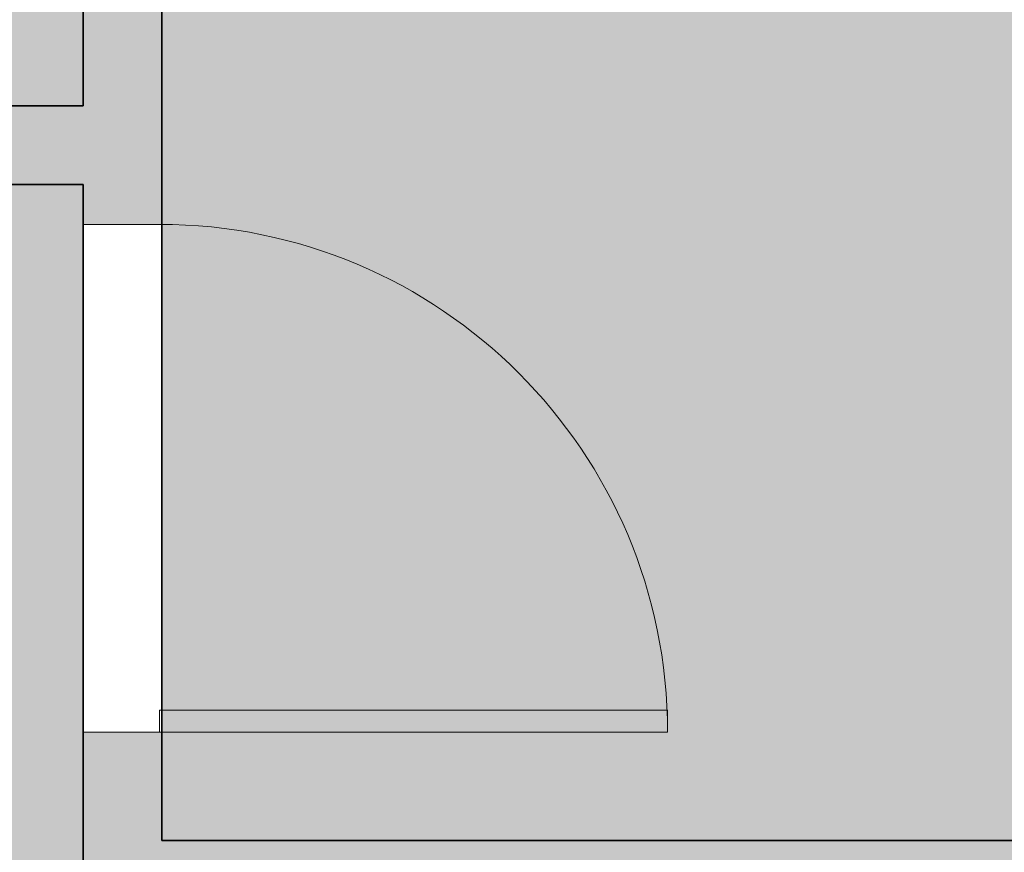
# Model space of a CAD drawing. Units: inches. Extents: x 1316 to 1777, y 813 to 1650.
# Tile 18 of 22: x 1567 to 1623, y 1434 to 1481. Entities that reach past the tile are written whole.
import ezdxf

# ---------------------------------------------------------------- set-up
doc = ezdxf.new("R2010")
doc.units = ezdxf.units.IN
doc.header["$MEASUREMENT"] = 0
for name, color, linetype, lineweight in [('A-DOOR', 4, 'Continuous', 18), ('A-WALL-PATT', 250, 'Continuous', 13), ('walls', 250, 'Continuous', 35)]:
    doc.layers.add(name, color=color, linetype=linetype, lineweight=lineweight)
doc.layers.add('A-FLOR-PATT', color=254, linetype='Continuous', lineweight=13, true_color=0xfeeab9)

# ---------------------------------------------------------------- blocks, each defined once
blk = doc.blocks.new('*U15')
for p, q in [((0, 0), (0, -6)), ((40, 0), (40, -6))]:
    blk.add_line(p, q)
blk.add_lwpolyline([(0, 0), (0, 40), (1.75, 40), (1.75, 0)], close=True)
blk.add_arc((0, 0), 40, 0, 90)

msp = doc.modelspace()

# ---------------------------------------------------------------- hatches: boundary and pattern name
at = {"layer": 'A-FLOR-PATT'}
h = msp.add_hatch(color=256, dxfattribs=at)
h.dxf.hatch_style = 1
h.paths.add_polyline_path([(1704.173, 1566.369), (1574.845, 1566.369), (1574.845, 1434.369), (1704.173, 1434.369)])
h.paths.add_polyline_path([(1630.932, 1542.856), (1660.956, 1542.856), (1660.956, 1535.716), (1688.427, 1535.716), (1688.322, 1546.604), (1686.085, 1547.859), (1686.091, 1547.88), (1685.166, 1550.963), (1681.619, 1555.397), (1678.246, 1552.474), (1678.253, 1552.433), (1678.187, 1552.423), (1681.619, 1555.397), (1683.601, 1556.058), (1683.639, 1556.172), (1683.764, 1556.112), (1686.94, 1557.171), (1688.039, 1558.585), (1688.034, 1558.699), (1688.108, 1558.672), (1686.969, 1557.208), (1686.965, 1557.18), (1681.619, 1555.397), (1682.039, 1554.872), (1682.12, 1554.846), (1682.107, 1554.788), (1685.145, 1550.989), (1685.188, 1550.977), (1685.173, 1550.941), (1685.764, 1548.971), (1688.364, 1547.814), (1702.185, 1547.814), (1702.301, 1535.716), (1702.301, 1481.716), (1702.418, 1469.617), (1688.544, 1469.617), (1688.427, 1481.716), (1660.956, 1481.716), (1660.956, 1470.853), (1630.932, 1470.853)], flags=16)
h.paths.add_polyline_path([(1624.931, 1450.279), (1703.919, 1450.279), (1703.919, 1436.32), (1703.919, 1435.026), (1624.931, 1435.026), (1624.931, 1435.469)], flags=16)
h.paths.add_polyline_path([(1624.931, 1443.714), (1625.995, 1443.714), (1625.995, 1449.229), (1626.752, 1449.229), (1626.752, 1443.714), (1628.114, 1443.714), (1628.114, 1449.229), (1628.871, 1449.229), (1628.871, 1443.714), (1630.502, 1443.714), (1630.502, 1449.229), (1631.259, 1449.229), (1631.259, 1443.714), (1632.968, 1443.714), (1632.968, 1449.229), (1633.724, 1449.229), (1633.724, 1443.714), (1638.318, 1443.714), (1641.013, 1449.6), (1641.689, 1449.29), (1639.136, 1443.714), (1640.128, 1443.714), (1642.823, 1449.6), (1643.499, 1449.29), (1640.945, 1443.714), (1642.323, 1443.714), (1645.018, 1449.6), (1645.694, 1449.29), (1643.141, 1443.714), (1647.035, 1443.714), (1647.035, 1449.229), (1647.792, 1449.229), (1647.792, 1443.714), (1649.606, 1443.714), (1649.606, 1449.229), (1650.363, 1449.229), (1650.363, 1443.714), (1652.865, 1443.714), (1652.865, 1449.229), (1653.621, 1449.229), (1653.621, 1443.714), (1657.035, 1443.714), (1657.035, 1449.229), (1657.792, 1449.229), (1657.792, 1443.714), (1660.083, 1443.714), (1660.083, 1449.229), (1660.839, 1449.229), (1660.839, 1443.714), (1662.605, 1443.714), (1662.605, 1449.229), (1663.362, 1449.229), (1663.362, 1443.714), (1667.702, 1443.714), (1667.702, 1449.229), (1668.459, 1449.229), (1668.459, 1443.714), (1671.655, 1443.714), (1670.316, 1449.229), (1671.051, 1449.407), (1672.434, 1443.714), (1679.696, 1443.714), (1680.179, 1449.244), (1680.933, 1449.178), (1680.455, 1443.714), (1683.5, 1443.714), (1682.225, 1448.723), (1682.959, 1448.91), (1684.281, 1443.714), (1688.219, 1443.714), (1688.219, 1449.229), (1688.976, 1449.229), (1688.976, 1443.714), (1690.482, 1443.714), (1690.482, 1449.229), (1691.239, 1449.229), (1691.239, 1443.714), (1692.488, 1443.714), (1692.488, 1449.229), (1693.245, 1449.229), (1693.245, 1443.714), (1695.009, 1443.714), (1695.009, 1449.229), (1695.766, 1449.229), (1695.766, 1443.714), (1701.029, 1443.714), (1700.875, 1443.379), (1695.766, 1443.379), (1695.766, 1435.872), (1695.009, 1435.872), (1695.009, 1443.379), (1693.245, 1443.379), (1693.245, 1435.872), (1692.488, 1435.872), (1692.488, 1443.379), (1691.239, 1443.379), (1691.239, 1435.872), (1690.482, 1435.872), (1690.482, 1443.379), (1688.976, 1443.379), (1688.976, 1435.872), (1688.219, 1435.872), (1688.219, 1443.379), (1684.366, 1443.379), (1686.252, 1435.965), (1685.518, 1435.779), (1683.585, 1443.379), (1680.426, 1443.379), (1679.77, 1435.872), (1679.016, 1435.938), (1679.666, 1443.379), (1677.602, 1443.379), (1677.602, 1435.46), (1676.845, 1435.46), (1676.845, 1443.379), (1672.515, 1443.379), (1674.202, 1436.427), (1673.467, 1436.249), (1671.736, 1443.379), (1668.459, 1443.379), (1668.459, 1435.872), (1667.702, 1435.872), (1667.702, 1443.379), (1663.362, 1443.379), (1663.362, 1435.872), (1662.605, 1435.872), (1662.605, 1443.379), (1660.839, 1443.379), (1660.839, 1435.872), (1660.083, 1435.872), (1660.083, 1443.379), (1657.792, 1443.379), (1657.792, 1435.872), (1657.035, 1435.872), (1657.035, 1443.379), (1653.621, 1443.379), (1653.621, 1435.872), (1652.865, 1435.872), (1652.865, 1443.379), (1650.363, 1443.379), (1650.363, 1435.872), (1649.606, 1435.872), (1649.606, 1443.379), (1647.792, 1443.379), (1647.792, 1435.872), (1647.035, 1435.872), (1647.035, 1443.379), (1642.988, 1443.379), (1639.39, 1435.522), (1638.715, 1435.832), (1642.17, 1443.379), (1640.792, 1443.379), (1637.195, 1435.522), (1636.519, 1435.832), (1639.974, 1443.379), (1638.983, 1443.379), (1635.385, 1435.522), (1634.709, 1435.832), (1638.165, 1443.379), (1633.724, 1443.379), (1633.724, 1435.872), (1632.968, 1435.872), (1632.968, 1443.379), (1631.259, 1443.379), (1631.259, 1435.872), (1630.502, 1435.872), (1630.502, 1443.379), (1628.871, 1443.379), (1628.871, 1435.872), (1628.114, 1435.872), (1628.114, 1443.379), (1626.752, 1443.379), (1626.752, 1435.872), (1625.995, 1435.872), (1625.995, 1443.379), (1624.931, 1443.379)], flags=0)
h.paths.add_polyline_path([(1683.839, 1491.517), (1691.022, 1491.517), (1691.071, 1491.582), (1691.071, 1529.618), (1699.231, 1529.618), (1699.231, 1513.795), (1691.071, 1513.795), (1691.071, 1507.34), (1699.231, 1507.34), (1699.231, 1491.517), (1691.022, 1491.517), (1683.839, 1481.774)], flags=0)
h.paths.add_polyline_path([(1691.015, 1475.341, -1), (1699.947, 1475.341, -1)], flags=0)
h.paths.add_polyline_path([(1690.898, 1541.439, -1), (1699.83, 1541.439, -1)], flags=0)
h.paths.add_polyline_path([(1505.845, 1469.591), (1505.845, 1566.369), (1386.064, 1566.369), (1386.064, 1450.329), (1465.697, 1450.329), (1465.697, 1449.245), (1466.177, 1449.025), (1465.697, 1447.977), (1465.697, 1436.055), (1465.697, 1434.369), (1505.845, 1434.369), (1505.845, 1440.551), (1476.949, 1440.551), (1476.949, 1441.822), (1476.977, 1441.822, -0.400014)])
edge = h.paths.add_edge_path(flags=16)
edge.add_spline(control_points=[(1456.973, 1471.794), (1457.023, 1471.721), (1457.138, 1471.554), (1456.942, 1471.242), (1456.67, 1470.851), (1456.943, 1470.632), (1457.081, 1470.522)], knot_values=[0, 0, 0, 0, 0.352144, 0.802463, 1.439322, 2.0926, 2.0926, 2.0926, 2.0926], degree=3, periodic=0)
edge.add_spline(control_points=[(1457.325, 1471.794), (1457.375, 1471.721), (1457.49, 1471.554), (1457.294, 1471.242), (1457.022, 1470.851), (1457.295, 1470.632), (1457.433, 1470.522)], knot_values=[0, 0, 0, 0, 0.352144, 0.802463, 1.439322, 2.0926, 2.0926, 2.0926, 2.0926], degree=3, periodic=0)
edge = h.paths.add_edge_path(flags=16)
edge.add_line((1429.513, 1471.794), (1429.513, 1482.657))
edge.add_line((1429.513, 1482.657), (1402.042, 1482.657))
edge.add_line((1402.042, 1482.657), (1401.925, 1470.559))
edge.add_line((1401.925, 1470.559), (1388.051, 1470.559))
edge.add_line((1388.051, 1470.559), (1388.167, 1482.657))
edge.add_line((1388.167, 1482.657), (1388.167, 1536.657))
edge.add_line((1388.167, 1536.657), (1388.284, 1548.755))
edge.add_line((1388.284, 1548.755), (1402.158, 1548.755))
edge.add_line((1402.158, 1548.755), (1402.042, 1536.657))
edge.add_line((1402.042, 1536.657), (1429.513, 1536.657))
edge.add_line((1429.513, 1536.657), (1429.513, 1543.797))
edge.add_line((1429.513, 1543.797), (1456.932, 1543.797))
edge.add_spline(control_points=[(1456.932, 1543.797), (1456.987, 1543.874), (1457.108, 1544.044), (1456.911, 1544.361), (1456.638, 1544.752), (1456.911, 1544.971), (1457.049, 1545.082)], knot_values=[0, 0, 0, 0, 0.373994, 0.824314, 1.461173, 2.114451, 2.114451, 2.114451, 2.114451], degree=3, periodic=0)
edge.add_spline(control_points=[(1457.401, 1545.082), (1457.263, 1544.971), (1456.99, 1544.752), (1457.263, 1544.361), (1457.46, 1544.044), (1457.339, 1543.874), (1457.284, 1543.797)], knot_values=[0, 0, 0, 0, 0.653278, 1.290138, 1.740457, 2.114451, 2.114451, 2.114451, 2.114451], degree=3, periodic=0)
edge.add_line((1457.284, 1543.797), (1459.536, 1543.797))
edge.add_line((1459.536, 1543.797), (1459.536, 1471.794))
edge.add_line((1459.536, 1471.794), (1429.513, 1471.794))
h.paths.add_polyline_path([(1406.63, 1482.715), (1399.446, 1492.458), (1399.398, 1492.458), (1391.238, 1492.458), (1391.238, 1508.281), (1399.398, 1508.281), (1399.398, 1514.736), (1391.238, 1514.736), (1391.238, 1530.559), (1399.398, 1530.559), (1399.398, 1492.524), (1399.446, 1492.458), (1406.63, 1492.458)], flags=0)
h.paths.add_polyline_path([(1399.454, 1476.282, -1), (1390.522, 1476.282, -1)], flags=0)
h.paths.add_polyline_path([(1390.638, 1542.38, -1), (1399.571, 1542.38, -1)], flags=0)
h.paths.add_polyline_path([(1487.293, 1548.286), (1487.08, 1548.252), (1487.104, 1547.964)], flags=16)
h.paths.add_polyline_path([(1491.493, 1552.843), (1490.887, 1552.654), (1490.949, 1552.372)], flags=16)
h.paths.add_polyline_path([(1489.966, 1554.409), (1489.859, 1554.561), (1489.718, 1554.445)], flags=16)
h.paths.add_polyline_path([(1497.301, 1546.483), (1497.294, 1546.462), (1497.309, 1546.453)], flags=16)
h.paths.add_polyline_path([(1496.386, 1549.553), (1492.828, 1554), (1492.655, 1554.939), (1492.454, 1555.029), (1492.589, 1555.296), (1491.806, 1559.547), (1491.869, 1559.506), (1491.824, 1559.451), (1492.828, 1554), (1494.81, 1554.661), (1494.848, 1554.774), (1494.973, 1554.715), (1496.01, 1555.061), (1496.078, 1555.314), (1496.341, 1555.171), (1498.15, 1555.774), (1499.249, 1557.187), (1499.243, 1557.301), (1499.317, 1557.275), (1498.179, 1555.811), (1498.174, 1555.782), (1492.828, 1554), (1493.249, 1553.474), (1493.33, 1553.449), (1493.316, 1553.39), (1495.203, 1551.032), (1495.702, 1550.957), (1495.574, 1550.568), (1496.354, 1549.592), (1496.397, 1549.58)], flags=16)
h.paths.add_polyline_path([(1486.021, 1555.224), (1485.958, 1555.549), (1483.595, 1557.912), (1483.28, 1557.859), (1483.243, 1558.264), (1486.27, 1555.237)], flags=16)
h.paths.add_polyline_path([(1505.845, 1469.591, 0.400014), (1476.977, 1441.822), (1505.845, 1441.822)], flags=17)
h = msp.add_hatch(color=256, dxfattribs=at)
h.dxf.hatch_style = 1
h.paths.add_polyline_path([(1561.016, 1510.243), (1561.016, 1510.275), (1562.477, 1510.275), (1562.477, 1476.879), (1562.477, 1471.869), (1529.081, 1471.869), (1529.081, 1476.879, -0.401453)])
h.paths.add_polyline_path([(1570.345, 1566.369), (1510.345, 1566.369), (1510.345, 1502.159), (1526.605, 1502.159), (1526.605, 1480.004), (1510.345, 1480.004), (1510.345, 1476.369), (1529.081, 1476.369), (1529.081, 1476.879, -0.401453), (1561.016, 1510.243), (1561.016, 1510.275), (1562.477, 1510.275), (1562.477, 1476.369), (1570.345, 1476.369)])
h.paths.add_polyline_path([(1528.659, 1540.982), (1528.659, 1542.825), (1529.12, 1552.041), (1528.659, 1552.041), (1528.659, 1553.884), (1529.12, 1553.884, -0.206081), (1535.571, 1559.041), (1535.571, 1561.257), (1534.65, 1561.257), (1534.65, 1562.179), (1532.806, 1562.179), (1532.806, 1563.1), (1543.866, 1563.1), (1543.866, 1562.179), (1542.023, 1562.179), (1542.023, 1561.257), (1541.101, 1561.257), (1541.101, 1559.041, -0.206081), (1547.552, 1553.884), (1548.013, 1553.884), (1548.013, 1552.041), (1547.552, 1552.041), (1547.552, 1542.825), (1548.013, 1542.825), (1548.013, 1540.982)], flags=16)
h.paths.add_polyline_path([(1704.173, 1429.869), (1602.173, 1429.869), (1602.173, 1408.281), (1631.07, 1408.281), (1631.07, 1407.011), (1631.042, 1407.011, -0.400014), (1602.173, 1379.241), (1602.173, 1369.869), (1625.31, 1369.869), (1625.31, 1385.783), (1647.465, 1385.783), (1647.465, 1369.869), (1704.173, 1369.869)])
h.paths.add_polyline_path([(1669.737, 1382.593), (1670.237, 1382.593), (1670.237, 1392.593), (1669.737, 1392.593), (1669.737, 1394.593), (1690.737, 1394.593), (1690.737, 1392.593), (1690.237, 1392.593), (1690.237, 1382.593), (1690.737, 1382.593), (1690.737, 1380.593), (1690.237, 1380.593, -0.206081), (1683.237, 1374.997), (1683.237, 1372.593), (1684.237, 1372.593), (1684.237, 1371.593), (1686.237, 1371.593), (1686.237, 1370.593), (1674.237, 1370.593), (1674.237, 1371.593), (1676.237, 1371.593), (1676.237, 1372.593), (1677.237, 1372.593), (1677.237, 1374.997, -0.206081), (1670.237, 1380.593), (1669.737, 1380.593)], flags=16)
h.paths.add_polyline_path([(1631.042, 1407.011), (1602.029, 1407.011), (1602.029, 1408.281), (1597.673, 1408.281), (1597.673, 1379.241), (1602.029, 1379.241, 0.401453)])
h = msp.add_hatch(color=256, dxfattribs=at)
h.dxf.hatch_style = 1
h.paths.add_polyline_path([(1567.673, 1281.369), (1651.673, 1281.369), (1651.673, 1365.369), (1597.673, 1365.369), (1597.673, 1429.869), (1570.345, 1429.869), (1570.345, 1471.869), (1510.345, 1471.869), (1510.345, 1429.869), (1444.564, 1429.869), (1444.564, 1322.882), (1444.564, 1300.088), (1510.564, 1300.088), (1510.564, 1295.094), (1510.564, 1240.869), (1386.064, 1240.869), (1386.064, 1171.185), (1400.961, 1171.185), (1400.961, 1106.742), (1386.064, 1106.742), (1386.064, 1072.869), (1510.564, 1072.869), (1510.564, 1040.173), (1541.068, 1040.173, -0.367085), (1572.764, 1069.547), (1572.764, 1069.579), (1574.225, 1069.579), (1574.225, 1040.173), (1616.037, 1040.173), (1616.037, 1086.627), (1616.037, 1103.705), (1613.066, 1105.235), (1616.037, 1106.686), (1616.037, 1123.869), (1567.673, 1123.869)])
h.paths.add_polyline_path([(1508.987, 1198.018), (1511.117, 1198.018), (1511.117, 1200.148), (1532.595, 1200.148), (1532.595, 1198.018), (1534.725, 1198.018), (1534.725, 1176.008), (1530.465, 1176.008), (1530.465, 1176.718), (1513.247, 1176.718), (1513.247, 1176.008), (1508.987, 1176.008)], flags=16)
h.paths.add_polyline_path([(1505.979, 1151.315), (1521.504, 1151.315), (1521.504, 1123.623), (1505.979, 1123.623)], flags=16)
h.paths.add_polyline_path([(1507.734, 1150.101, -1), (1506.932, 1150.101, -1)], flags=0)
h.paths.add_polyline_path([(1512.288, 1138.353), (1512.28, 1138.392), (1512.219, 1138.376)], flags=0)
h.paths.add_polyline_path([(1511.539, 1138.926), (1511.802, 1138.967), (1511.817, 1139.27), (1511.607, 1139.246)], flags=0)
h.paths.add_polyline_path([(1513.745, 1140.234), (1513.68, 1139.885), (1514.014, 1140.045), (1513.855, 1140.308)], flags=0)
h.paths.add_polyline_path([(1513.759, 1139.089), (1514.005, 1139.255), (1513.807, 1139.483), (1513.564, 1139.327)], flags=0)
h.paths.add_polyline_path([(1514.219, 1138.385), (1514.336, 1138.33), (1514.544, 1138.32), (1514.802, 1138.874), (1514.451, 1138.716)], flags=0)
h.paths.add_polyline_path([(1514.577, 1137.439), (1514.573, 1137.4), (1514.699, 1137.4), (1514.696, 1137.402)], flags=0)
h.paths.add_polyline_path([(1512.26, 1136.199), (1512.199, 1136.399), (1512.032, 1136.325), (1512.095, 1136.101), (1512.257, 1136.192)], flags=0)
h.paths.add_polyline_path([(1512.644, 1137.274), (1512.356, 1137.23), (1512.432, 1137.049), (1512.703, 1137.093)], flags=0)
h.paths.add_polyline_path([(1513.049, 1137.593), (1512.979, 1137.8), (1512.843, 1137.757), (1512.887, 1137.556)], flags=0)
h.paths.add_polyline_path([(1513.269, 1138.556), (1513.571, 1137.962), (1513.459, 1136.814), (1513.212, 1137.878), (1513.032, 1138.443)], flags=0)
h.paths.add_polyline_path([(1514.891, 1136.377), (1514.696, 1136.401), (1514.683, 1136.246), (1514.87, 1136.165)], flags=0)
h.paths.add_polyline_path([(1514.142, 1137.293), (1514.047, 1136.743), (1514.27, 1136.751), (1514.328, 1137.265)], flags=0)
h.paths.add_polyline_path([(1515.362, 1138.976), (1515.334, 1138.638), (1515.596, 1138.588), (1515.627, 1138.932)], flags=0)
h.paths.add_polyline_path([(1537.285, 1177.912), (1537.995, 1177.912), (1537.995, 1195.13), (1537.285, 1195.13), (1537.285, 1199.39), (1559.295, 1199.39), (1559.295, 1197.26), (1561.425, 1197.26), (1561.425, 1175.782), (1559.295, 1175.782), (1559.295, 1173.652), (1559.379, 1173.652), (1559.379, 1171.514), (1561.517, 1171.514), (1561.517, 1098.819), (1559.379, 1098.819), (1559.379, 1096.68), (1537.285, 1096.68), (1537.285, 1100.957), (1537.997, 1100.957), (1537.997, 1169.376), (1537.285, 1169.376), (1537.285, 1173.652)], flags=16)
h.paths.add_polyline_path([(1518.623, 1345.565), (1519.133, 1345.48), (1519.133, 1345.485), (1518.623, 1345.567)], flags=16)
h.paths.add_polyline_path([(1518.798, 1374.15), (1519.308, 1374.064), (1519.308, 1374.069), (1518.798, 1374.152)], flags=16)
h.paths.add_polyline_path([(1537.764, 1413.501), (1537.678, 1412.991), (1537.683, 1412.991), (1537.766, 1413.501)], flags=16)
h.paths.add_polyline_path([(1572.905, 1373.821), (1573.927, 1373.975), (1574.027, 1390.309), (1573.007, 1390.475), (1573.007, 1390.475)], flags=16)
h.paths.add_polyline_path([(1572.73, 1345.237), (1573.752, 1345.39), (1573.852, 1361.724), (1572.832, 1361.89), (1572.832, 1361.89)], flags=16)
h.paths.add_polyline_path([(1537.211, 1322.643), (1537.364, 1321.621), (1553.698, 1321.521), (1553.864, 1322.541)], flags=16)
h.paths.add_polyline_path([(1535.908, 1331.328), (1527.214, 1331.382), (1527.664, 1404.885), (1564.416, 1404.66), (1563.966, 1331.157), (1555.273, 1331.21), (1553.947, 1323.051), (1537.134, 1323.154)], flags=16)
h.paths.add_polyline_path([(1536.15, 1336.503), (1536.235, 1337.572), (1536.323, 1338.628), (1536.411, 1339.663), (1536.495, 1340.67), (1536.574, 1341.66), (1536.648, 1342.648), (1536.717, 1343.649), (1536.78, 1344.678), (1536.837, 1345.75), (1536.913, 1347.475), (1536.93, 1348.082), (1536.867, 1346.314), (1536.754, 1344.188), (1536.619, 1342.219), (1536.495, 1340.67), (1536.411, 1339.663), (1536.323, 1338.628), (1536.235, 1337.572), (1536.15, 1336.503), (1536.071, 1335.432), (1536.002, 1334.37), (1535.917, 1332.754), (1535.909, 1332.308), (1535.964, 1333.78), (1536.071, 1335.432)], flags=0)
h.paths.add_polyline_path([(1540.412, 1338.345), (1540.539, 1339.037), (1540.667, 1339.758), (1540.798, 1340.518), (1540.93, 1341.325), (1541.063, 1342.187), (1541.196, 1343.109), (1541.326, 1344.085), (1541.45, 1345.102), (1541.566, 1346.15), (1541.669, 1347.219), (1541.758, 1348.296), (1541.829, 1349.371), (1541.879, 1350.434), (1541.906, 1351.476), (1541.91, 1352.5), (1541.895, 1353.512), (1541.861, 1354.518), (1541.812, 1355.524), (1541.749, 1356.537), (1541.674, 1357.561), (1541.551, 1359.062), (1541.495, 1359.67), (1541.589, 1358.603), (1541.721, 1356.977), (1541.846, 1354.98), (1541.912, 1352.982), (1541.903, 1350.951), (1541.806, 1348.87), (1541.628, 1346.713), (1541.396, 1344.612), (1541.135, 1342.656), (1540.872, 1340.947), (1540.617, 1339.466), (1540.412, 1338.345), (1540.288, 1337.675), (1540.166, 1337.018), (1540.049, 1336.365), (1539.937, 1335.71), (1539.837, 1335.055), (1539.758, 1334.403), (1539.709, 1333.756), (1539.697, 1333.12), (1539.751, 1332.162), (1539.822, 1331.89), (1539.691, 1332.775), (1539.714, 1334.035), (1539.867, 1335.303), (1540.085, 1336.577), (1540.288, 1337.675)], flags=0)
h.paths.add_polyline_path([(1545.599, 1331.584), (1545.601, 1331.617), (1545.614, 1331.689), (1545.737, 1332.197), (1545.767, 1332.332), (1545.84, 1332.681), (1545.925, 1333.114), (1546.016, 1333.614), (1546.108, 1334.164), (1546.196, 1334.748), (1546.276, 1335.349), (1546.342, 1335.952), (1546.388, 1336.539), (1546.412, 1337.098), (1546.414, 1337.632), (1546.395, 1338.145), (1546.359, 1338.645), (1546.306, 1339.137), (1546.24, 1339.627), (1546.161, 1340.121), (1546.073, 1340.625), (1545.888, 1341.63), (1545.718, 1342.621), (1545.547, 1343.945), (1545.432, 1345.534), (1545.404, 1347.402), (1545.418, 1348.013), (1545.411, 1346.957), (1545.425, 1345.988), (1545.463, 1345.105), (1545.521, 1344.301), (1545.596, 1343.566), (1545.683, 1342.892), (1545.778, 1342.27), (1545.877, 1341.691), (1545.977, 1341.145), (1546.133, 1340.297), (1546.327, 1339.075), (1546.434, 1337.615), (1546.377, 1336.279), (1546.246, 1335.079), (1546.032, 1333.665), (1545.84, 1332.681), (1545.767, 1332.332)], flags=0)
h.paths.add_polyline_path([(1551.803, 1337.656), (1551.963, 1338.25), (1552.102, 1338.801), (1552.225, 1339.338), (1552.331, 1339.865), (1552.418, 1340.377), (1552.487, 1340.873), (1552.536, 1341.348), (1552.563, 1341.801), (1552.569, 1342.228), (1552.551, 1342.627), (1552.51, 1342.995), (1552.446, 1343.333), (1552.363, 1343.646), (1552.261, 1343.937), (1552.144, 1344.207), (1552.012, 1344.461), (1551.868, 1344.7), (1551.746, 1344.882), (1550.887, 1346.052), (1550.428, 1347.126), (1550.183, 1348.353), (1550.048, 1349.632), (1549.978, 1351.224), (1549.974, 1353.141), (1549.989, 1353.748), (1549.975, 1352.682), (1549.977, 1351.708), (1549.996, 1350.825), (1550.031, 1350.027), (1550.082, 1349.31), (1550.15, 1348.669), (1550.234, 1348.098), (1550.335, 1347.593), (1550.452, 1347.149), (1550.584, 1346.76), (1550.73, 1346.419), (1550.887, 1346.117), (1551.05, 1345.848), (1551.217, 1345.602), (1551.386, 1345.372), (1551.553, 1345.151), (1552, 1344.537), (1552.454, 1343.495), (1552.591, 1342.266), (1552.509, 1340.905), (1552.246, 1339.367), (1551.925, 1338.101), (1551.619, 1336.984), (1551.406, 1336.2), (1551.01, 1334.699), (1550.877, 1334.155), (1551.264, 1335.677), (1551.619, 1336.984)], flags=0)
h.paths.add_polyline_path([(1558.642, 1348.348), (1558.795, 1348.811), (1558.918, 1349.215), (1559.008, 1349.575), (1559.061, 1349.904), (1559.076, 1350.214), (1559.054, 1350.506), (1559.001, 1350.776), (1558.919, 1351.021), (1558.814, 1351.239), (1558.688, 1351.425), (1558.546, 1351.578), (1558.392, 1351.694), (1558.229, 1351.772), (1558.059, 1351.812), (1557.882, 1351.819), (1557.701, 1351.794), (1557.515, 1351.742), (1557.327, 1351.665), (1557.136, 1351.566), (1556.944, 1351.448), (1556.752, 1351.315), (1556.742, 1351.307), (1556.175, 1350.878), (1555.982, 1350.741), (1555.79, 1350.618), (1555.103, 1350.248), (1554.019, 1350.696), (1553.658, 1351.734), (1553.592, 1352.861), (1553.705, 1354.248), (1553.753, 1354.657), (1553.685, 1354.004), (1553.638, 1353.425), (1553.615, 1352.918), (1553.615, 1352.476), (1553.637, 1352.094), (1553.681, 1351.766), (1553.745, 1351.485), (1553.828, 1351.246), (1553.929, 1351.043), (1554.048, 1350.87), (1554.182, 1350.722), (1554.33, 1350.599), (1554.491, 1350.501), (1554.662, 1350.43), (1554.841, 1350.388), (1555.026, 1350.374), (1555.215, 1350.39), (1555.406, 1350.437), (1555.598, 1350.514), (1555.79, 1350.618), (1555.982, 1350.741), (1556.175, 1350.878), (1556.367, 1351.024), (1556.559, 1351.171), (1556.752, 1351.315), (1556.944, 1351.448), (1557.136, 1351.566), (1557.327, 1351.665), (1558.043, 1351.957), (1558.894, 1351.316), (1559.137, 1350.09), (1558.886, 1349.087), (1558.642, 1348.348), (1558.463, 1347.812), (1558.261, 1347.187), (1558.039, 1346.459), (1557.677, 1345.175), (1557.549, 1344.636), (1557.909, 1346.03), (1558.329, 1347.408)], flags=0)
h.paths.add_polyline_path([(1562.145, 1353.919), (1562.25, 1354.68), (1562.341, 1355.344), (1562.416, 1355.924), (1562.475, 1356.431), (1562.518, 1356.872), (1562.544, 1357.254), (1562.554, 1357.582), (1562.548, 1357.862), (1562.525, 1358.1), (1562.486, 1358.303), (1562.432, 1358.476), (1562.361, 1358.624), (1562.277, 1358.748), (1562.18, 1358.848), (1562.073, 1358.925), (1561.958, 1358.977), (1561.837, 1359.006), (1561.711, 1359.011), (1561.584, 1358.992), (1561.456, 1358.949), (1561.342, 1358.895), (1560.78, 1358.554), (1560.631, 1358.473), (1560.474, 1358.403), (1560.311, 1358.348), (1559.637, 1358.207), (1558.973, 1358.904), (1558.816, 1360.002), (1558.804, 1361.236), (1558.83, 1361.674), (1558.807, 1360.917), (1558.813, 1360.297), (1558.845, 1359.795), (1558.902, 1359.397), (1558.982, 1359.087), (1559.082, 1358.849), (1559.2, 1358.666), (1559.334, 1358.525), (1559.482, 1358.421), (1559.639, 1358.351), (1559.804, 1358.311), (1559.973, 1358.3), (1560.143, 1358.313), (1560.311, 1358.348), (1560.474, 1358.403), (1560.631, 1358.473), (1560.78, 1358.554), (1560.923, 1358.641), (1561.061, 1358.729), (1561.196, 1358.813), (1561.382, 1358.92), (1561.342, 1358.895), (1561.972, 1359.194), (1562.536, 1358.367), (1562.56, 1357.311), (1562.455, 1356.226), (1562.323, 1355.206), (1562.145, 1353.919), (1562.026, 1353.049), (1561.815, 1351.457), (1561.752, 1350.933), (1561.948, 1352.479)], flags=0)
h.paths.add_polyline_path([(1572.764, 1069.547, 0.367085), (1541.068, 1040.173), (1572.764, 1040.173)], flags=17)
h.paths.add_polyline_path([(1572.764, 1040.173), (1541.068, 1040.173, 0.029954), (1540.829, 1036.182), (1540.829, 1031.173), (1574.225, 1031.173), (1574.225, 1036.182), (1572.764, 1036.182)])
at = {"layer": 'A-WALL-PATT'}
h = msp.add_hatch(color=256, dxfattribs=at)
h.dxf.hatch_style = 1
h.paths.add_polyline_path([(1713.173, 1281.369), (1656.173, 1281.369), (1656.173, 1298.258), (1651.673, 1298.258), (1651.673, 1281.369), (1567.673, 1281.369), (1567.673, 1266.995), (1572.173, 1266.995), (1572.173, 1276.869), (1704.173, 1276.869), (1704.173, 1132.869), (1608.64, 1132.869), (1608.64, 1123.869), (1704.173, 1123.869), (1704.173, 1040.173), (1652.869, 1040.173), (1652.869, 1031.173), (1713.173, 1031.173), (1713.173, 1040.173)])
h.paths.add_polyline_path([(1572.173, 1237.955), (1567.673, 1237.955), (1567.673, 1123.869), (1583.146, 1123.869), (1583.146, 1132.869), (1572.173, 1132.869)], flags=17)
h.paths.add_polyline_path([(1510.345, 1566.369), (1524.171, 1566.369), (1524.171, 1571.985), (1524.171, 1575.369), (1445.955, 1575.369), (1445.955, 1566.369), (1505.845, 1566.369), (1505.845, 1469.591), (1510.345, 1469.591), (1510.345, 1471.869), (1529.081, 1471.869), (1529.081, 1476.369), (1510.345, 1476.369)])
h.paths.add_polyline_path([(1609.722, 1575.369), (1545.119, 1575.369), (1545.119, 1566.369), (1570.345, 1566.369), (1570.345, 1476.369), (1562.477, 1476.369), (1562.477, 1471.869), (1570.345, 1471.869), (1570.345, 1469.591), (1574.845, 1469.591), (1574.845, 1566.369), (1609.722, 1566.369)])
h.paths.add_polyline_path([(1713.173, 1575.369), (1655.233, 1575.369), (1655.233, 1566.369), (1704.173, 1566.369), (1704.173, 1434.369), (1574.845, 1434.369), (1574.845, 1440.551), (1574.701, 1440.551), (1570.345, 1440.551), (1570.345, 1429.869), (1597.673, 1429.869), (1597.673, 1408.281), (1602.173, 1408.281), (1602.173, 1429.869), (1704.173, 1429.869), (1704.173, 1410.704), (1707.375, 1410.704), (1713.173, 1410.704)])
h.paths.add_polyline_path([(1713.173, 1383.676), (1704.173, 1383.676), (1704.173, 1369.869), (1602.173, 1369.869), (1602.173, 1379.241), (1597.673, 1379.241), (1597.673, 1365.369), (1713.173, 1365.369)])
h.paths.add_polyline_path([(1444.564, 1429.869), (1510.345, 1429.869), (1510.345, 1440.551), (1505.845, 1440.551), (1505.845, 1434.369), (1386.064, 1434.369), (1386.064, 1566.369), (1400.445, 1566.369), (1400.445, 1575.369), (1377.064, 1575.369), (1377.064, 1412.813), (1380.509, 1412.813), (1386.064, 1412.813), (1386.064, 1429.869), (1440.064, 1429.869), (1440.064, 1401.229), (1444.564, 1401.229)])
h.paths.add_polyline_path([(1444.564, 1372.189), (1440.064, 1372.189), (1440.064, 1369.869), (1386.064, 1369.869), (1386.064, 1378.758), (1377.064, 1378.758), (1377.064, 1349.201), (1381.118, 1349.201), (1386.064, 1349.201), (1386.064, 1365.369), (1440.064, 1365.369), (1440.064, 1322.882), (1444.564, 1322.882)])
h.paths.add_polyline_path([(1510.564, 1295.094), (1506.064, 1295.094), (1506.064, 1245.369), (1386.064, 1245.369), (1386.064, 1272.582), (1377.064, 1272.582), (1377.064, 1212.905), (1380.1, 1212.905), (1386.064, 1212.905), (1386.064, 1240.869), (1510.564, 1240.869)])
h.paths.add_polyline_path([(1386.064, 1163.761), (1377.064, 1163.761), (1377.064, 1063.869), (1419.363, 1063.869), (1419.363, 1072.869), (1386.064, 1072.869)])
h.paths.add_polyline_path([(1510.564, 1072.869), (1469.381, 1072.869), (1469.381, 1063.869), (1501.564, 1063.869), (1501.564, 1033.023), (1501.564, 1031.173), (1540.829, 1031.173), (1540.829, 1036.182, -0.029954), (1541.068, 1040.173), (1510.564, 1040.173)])
h.paths.add_polyline_path([(1607.369, 1040.173), (1574.225, 1040.173), (1574.225, 1036.182), (1574.225, 1031.173), (1607.369, 1031.173)], flags=17)
h.paths.add_polyline_path([(1637.054, 1040.173), (1624.706, 1040.173), (1624.706, 1031.173), (1637.054, 1031.173)], flags=17)

# ---------------------------------------------------------------- linework, layer by layer
at = {"layer": 'walls'}
for p, q in [((1570.345, 1566.369), (1570.345, 1476.369)), ((1574.845, 1566.369), (1574.845, 1434.369)), ((1510.345, 1476.369), (1570.345, 1476.369)), ((1510.345, 1471.869), (1570.345, 1471.869)), ((1570.345, 1471.869), (1570.345, 1429.869)), ((1574.845, 1434.369), (1704.173, 1434.369))]:
    msp.add_line(p, q, dxfattribs=at)

# ---------------------------------------------------------------- block references
at = {"layer": 'A-DOOR', "xscale": -0.7260080760128325, "yscale": 0.7260080760128325, "zscale": 0.7260080760128325, "rotation": 270}
msp.add_blockref('*U15', (1574.701, 1440.551), dxfattribs=at)

doc.saveas('drawing.dxf')
